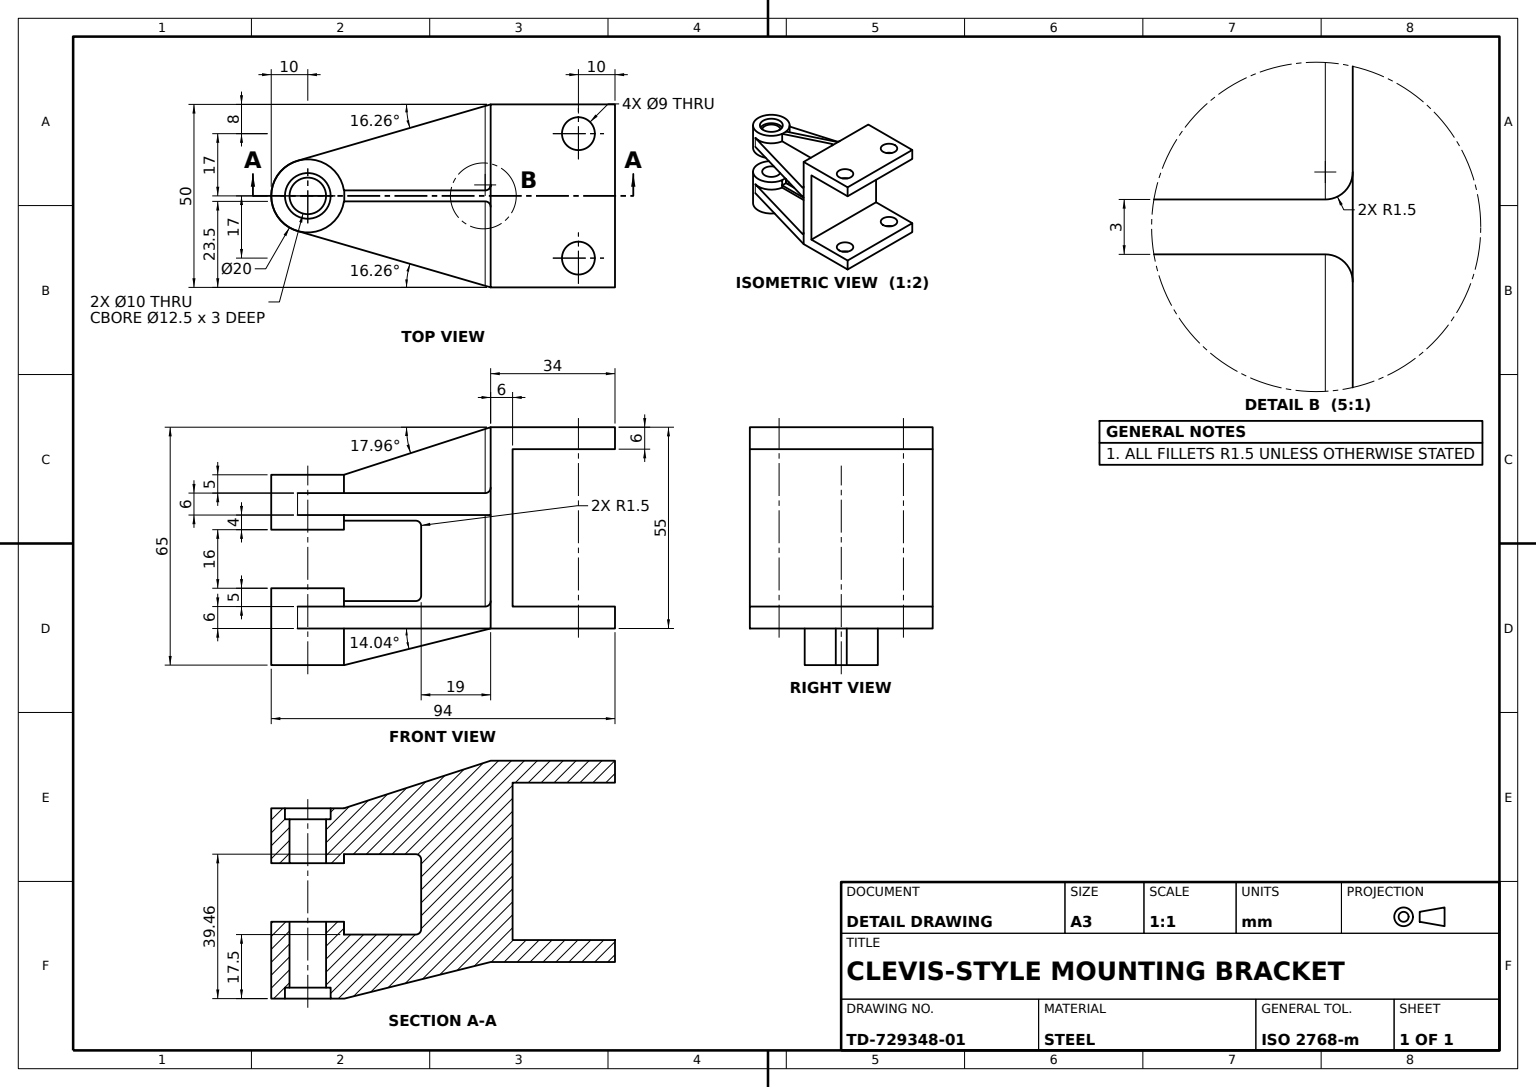
from build123d import *

# Parameters (mm, degrees)
U_CHANNEL_BASE_DEPTH             = 25
UPPER_LUG_BOSS_SKETCH_20_R       = 10
UPPER_LUG_BOSS_20_DEPTH          = 10
UPPER_START                      = 5
UPPER_LUG_PAD_SKETCH_R           = 10
UPPER_LUG_PAD_DEPTH              = 5
UPPER_COUNTERBORE_SKETCH_12_5_R  = 6.25
UPPER_COUNTERBORE_12_5_DEPTH     = 3
UPPER_LUG_HOLE_SKETCH_10_R       = 5
UPPER_LUG_HOLE_10_DEPTH          = 12
LOWER_START                      = -11
LOWER_LUG_PAD_SKETCH_R           = 10
LOWER_LUG_PAD_DEPTH              = 11
LOWER_LUG_BOSS_SKETCH_20_R       = 10
LOWER_LUG_BOSS_20_DEPTH          = 10
LOWER_START_2                    = -3
LOWER_COUNTERBORE_SKETCH_12_5_R  = 6.25
LOWER_COUNTERBORE_12_5_DEPTH     = 3
LOWER_START_3                    = -18
LOWER_LUG_HOLE_SKETCH_10_R       = 5
LOWER_LUG_HOLE_10_DEPTH          = 18
UPPER_GUSSET_DEPTH               = 6
UPPER_GUSSET_TRIM_DEPTH          = 6
LOWER_GUSSET_DEPTH               = 6
LOWER_GUSSET_TRIM_DEPTH          = 6
BACK_PLATE_DEPTH                 = 1.5
BACK_PLATE_LOWER_RELIEF_DEPTH    = 3
LOWER_LUG_RELIEF_SKETCH_W        = 3
LOWER_LUG_RELIEF_SKETCH_H        = 5
LOWER_LUG_RELIEF_DEPTH           = 3
BACK_PLATE_UPPER_RELIEF_SKETCH_W = 40.123603225
BACK_PLATE_UPPER_RELIEF_SKETCH_H = 13
BACK_PLATE_UPPER_RELIEF_DEPTH    = 3
BACK_PLATE_EDGE_TRIM_SKETCH_W    = 21.123603225
BACK_PLATE_EDGE_TRIM_SKETCH_H    = 21.964107992
BACK_PLATE_EDGE_TRIM_DEPTH       = 3
WEB_SKETCH_W                     = 40.123603225
WEB_SKETCH_H                     = 3
WEB_DEPTH                        = 18
WEB_CHAMFER_CUT_DEPTH            = 3
WEB_FACE_TRIM_SKETCH_W           = 3
WEB_FACE_TRIM_SKETCH_H           = 13
WEB_FACE_TRIM_0_1_DEPTH          = 0.1
FLANGE_MOUNTING_HOLES_SKETCH_R   = 4.5
FLANGE_MOUNTING_HOLES_4X_DEPTH   = 59.1
EDGE_FILLET_R1_5_R               = 1.5


with BuildPart() as part:
    # U-Channel Profile Sketch → U-Channel Base (new, symmetric)
    with BuildSketch(Plane.XY):
        Polygon((0, 37.5), (0, 19.5), (-50, 19.5), (-50, 13.5), (0, 13.5), (0, -11.5), (-50, -11.5), (-50, -17.5), (0, -17.5), (34, -17.5), (34, -11.5), (6, -11.5), (6, 31.5), (34, 31.5), (34, 37.5), align=None)
    extrude(amount=U_CHANNEL_BASE_DEPTH, both=True)

    # Upper Lug Boss Sketch Ø20 → Upper Lug Boss Ø20 (add)
    with BuildSketch(Plane(origin=(0, 19.5, 0), x_dir=(1, 0, 0), z_dir=(0, 1, 0))):
        with Locations(Location((-50, 0, 0), (0, 0, 180))):
            Circle(UPPER_LUG_BOSS_SKETCH_20_R)
    extrude(amount=-UPPER_LUG_BOSS_20_DEPTH)

    # Upper Lug Pad Sketch → Upper Lug Pad (add)
    with BuildSketch(Plane(origin=(0, 19.5, 0), x_dir=(1, 0, 0), z_dir=(0, 1, 0)).offset(UPPER_START)):
        with Locations(Location((-50, 0, 0), (0, 0, 180))):
            Circle(UPPER_LUG_PAD_SKETCH_R)
    extrude(amount=-UPPER_LUG_PAD_DEPTH)

    # Upper Counterbore Sketch Ø12.5 → Upper Counterbore Ø12.5 (cut)
    with BuildSketch(Plane(origin=(0, 24.5, 0), x_dir=(1, 0, 0), z_dir=(0, 1, 0))):
        with Locations(Location((-50, 0, 0), (0, 0, 180))):
            Circle(UPPER_COUNTERBORE_SKETCH_12_5_R)
    extrude(amount=-UPPER_COUNTERBORE_12_5_DEPTH, mode=Mode.SUBTRACT)

    # Upper Lug Hole Sketch Ø10 → Upper Lug Hole Ø10 (cut)
    with BuildSketch(Plane(origin=(0, 21.5, 0), x_dir=(1, 0, 0), z_dir=(0, 1, 0))):
        with Locations(Location((-50, 0, 0), (0, 0, 180))):
            Circle(UPPER_LUG_HOLE_SKETCH_10_R)
    extrude(amount=-UPPER_LUG_HOLE_10_DEPTH, mode=Mode.SUBTRACT)

    # Lower Lug Pad Sketch → Lower Lug Pad (add)
    with BuildSketch(Plane.XZ.offset(17.5).offset(LOWER_START)):
        with Locations(Location((-50, 0, 0), (0, 0, 180))):
            Circle(LOWER_LUG_PAD_SKETCH_R)
    extrude(amount=LOWER_LUG_PAD_DEPTH)

    # Lower Lug Boss Sketch Ø20 → Lower Lug Boss Ø20 (add)
    with BuildSketch(Plane.XZ.offset(17.5)):
        with Locations(Location((-50, 0, 0), (0, 0, 180))):
            Circle(LOWER_LUG_BOSS_SKETCH_20_R)
    extrude(amount=LOWER_LUG_BOSS_20_DEPTH)

    # Lower Counterbore Sketch Ø12.5 → Lower Counterbore Ø12.5 (cut)
    with BuildSketch(Plane.XZ.offset(27.5).offset(LOWER_START_2)):
        with Locations(Location((-50, 0, 0), (0, 0, 180))):
            Circle(LOWER_COUNTERBORE_SKETCH_12_5_R)
    extrude(amount=LOWER_COUNTERBORE_12_5_DEPTH, mode=Mode.SUBTRACT)

    # Lower Lug Hole Sketch Ø10 → Lower Lug Hole Ø10 (cut)
    with BuildSketch(Plane.XZ.offset(24.5).offset(LOWER_START_3)):
        with Locations(Location((-50, 0, 0), (0, 0, 180))):
            Circle(LOWER_LUG_HOLE_SKETCH_10_R)
    extrude(amount=LOWER_LUG_HOLE_10_DEPTH, mode=Mode.SUBTRACT)

    # Upper Gusset Sketch → Upper Gusset (add)
    with BuildSketch(Plane(origin=(0, 19.5, 0), x_dir=(1, 0, 0), z_dir=(0, 1, 0))):
        Polygon((0, 25), (-50, 10.416666667), (-50, 10), (-52.8, 9.6), (-52.8, 25), align=None)
        Polygon((-52.8, -9.6), (-52.8, -25), (0, -25), (-50, -10.416666667), (-50, -10), align=None)
    extrude(amount=-UPPER_GUSSET_DEPTH)

    # Upper Gusset Trim Sketch → Upper Gusset Trim (cut)
    with BuildSketch(Plane(origin=(0, 19.5, 0), x_dir=(1, 0, 0), z_dir=(0, 1, 0))):
        Polygon((0, 25), (-52.8, 9.6), (-52.8, 25), align=None)
        Polygon((0, -25), (-52.8, -9.6), (-52.8, -25), align=None)
    extrude(amount=-UPPER_GUSSET_TRIM_DEPTH, mode=Mode.SUBTRACT)

    # Lower Gusset Sketch → Lower Gusset (add)
    with BuildSketch(Plane.XZ.offset(17.5)):
        Polygon((0, 25), (-50, 10.416666667), (-50, 10), (-52.8, 9.6), (-52.8, 25), align=None)
        Polygon((0, -25), (-50, -10.416666667), (-50, -10), (-52.8, -9.6), (-52.8, -25), align=None)
    extrude(amount=-LOWER_GUSSET_DEPTH)

    # Lower Gusset Trim Sketch → Lower Gusset Trim (cut)
    with BuildSketch(Plane.XZ.offset(17.5)):
        Polygon((0, 25), (-52.8, 9.6), (-52.8, 25), align=None)
        Polygon((0, -25), (-52.8, -9.6), (-52.8, -25), align=None)
    extrude(amount=-LOWER_GUSSET_TRIM_DEPTH, mode=Mode.SUBTRACT)


with BuildPart() as body_2:
    # Back Plate Sketch → Back Plate (new, symmetric)
    with BuildSketch(Plane.XY):
        Polygon((0, 0), (0, 32.5), (-40.123603225, 32.5), (-40.123603225, -32.5), (0, -32.5), align=None)
    extrude(amount=BACK_PLATE_DEPTH, both=True)

    # Back Plate Lower Relief Sketch → Back Plate Lower Relief (cut)
    with BuildSketch(Plane.XY.offset(1.5)):
        Polygon((-40, -27.5), (0, -17.5), (0, -32.5), (-40.123603225, -32.5), align=None)
    extrude(amount=-BACK_PLATE_LOWER_RELIEF_DEPTH, mode=Mode.SUBTRACT)

    # Lower Lug Relief Sketch → Lower Lug Relief (cut)
    with BuildSketch(Plane.ZY.offset(40.123603225)):
        with Locations((0, -30)):
            Rectangle(LOWER_LUG_RELIEF_SKETCH_W, LOWER_LUG_RELIEF_SKETCH_H)
    extrude(amount=-LOWER_LUG_RELIEF_DEPTH, mode=Mode.SUBTRACT)


with BuildPart() as back_plate_upper_relief_tool:
    # Back Plate Upper Relief Sketch → Back Plate Upper Relief (new body)
    with BuildSketch(Plane.XY.offset(1.5)):
        with Locations((-20.061801613, 26)):
            Rectangle(BACK_PLATE_UPPER_RELIEF_SKETCH_W, BACK_PLATE_UPPER_RELIEF_SKETCH_H)
    extrude(amount=-BACK_PLATE_UPPER_RELIEF_DEPTH)


with BuildPart() as part_1:
    add(part.part)

    # Back Plate Upper Relief: cut by back_plate_upper_relief_tool
    add(back_plate_upper_relief_tool.part, mode=Mode.SUBTRACT)


with BuildPart() as body_2_1:
    add(body_2.part)

    # Back Plate Upper Relief: cut by back_plate_upper_relief_tool
    add(back_plate_upper_relief_tool.part, mode=Mode.SUBTRACT)


with BuildPart() as back_plate_edge_trim_tool:
    # Back Plate Edge Trim Sketch → Back Plate Edge Trim (new body)
    with BuildSketch(Plane.XY.offset(1.5)):
        with Locations((-29.561801613, 0.982053996)):
            Rectangle(BACK_PLATE_EDGE_TRIM_SKETCH_W, BACK_PLATE_EDGE_TRIM_SKETCH_H)
    extrude(amount=-BACK_PLATE_EDGE_TRIM_DEPTH)


with BuildPart() as part_2:
    add(part_1.part)

    # Back Plate Edge Trim: cut by back_plate_edge_trim_tool
    add(back_plate_edge_trim_tool.part, mode=Mode.SUBTRACT)



with BuildPart() as body_2_2:
    add(body_2_1.part)

    # Back Plate Edge Trim: cut by back_plate_edge_trim_tool
    add(back_plate_edge_trim_tool.part, mode=Mode.SUBTRACT)


with BuildPart() as part_3:
    add(part_2.part)

    add(body_2_2.part)  # Web merges body 2
    # Web Sketch → Web (add)
    with BuildSketch(Plane(origin=(0, 19.5, 0), x_dir=(1, 0, 0), z_dir=(0, 1, 0))):
        with Locations((-20.061801613, 0)):
            Rectangle(WEB_SKETCH_W, WEB_SKETCH_H)
    extrude(amount=WEB_DEPTH)

    # Web Chamfer Cut Sketch → Web Chamfer Cut (cut)
    with BuildSketch(Plane.XY.offset(1.5)):
        Polygon((0, 37.5), (-40.113140033, 24.5), (-40.123603225, 37.5), align=None)
    extrude(amount=-WEB_CHAMFER_CUT_DEPTH, mode=Mode.SUBTRACT)

    # Web Face Trim Sketch → Web Face Trim 0.1 (cut)
    with BuildSketch(Plane.ZY.offset(40.123603225)):
        with Locations((0, 31)):
            Rectangle(WEB_FACE_TRIM_SKETCH_W, WEB_FACE_TRIM_SKETCH_H)
    extrude(amount=-WEB_FACE_TRIM_0_1_DEPTH, mode=Mode.SUBTRACT)

    # Flange Mounting Holes Sketch → Flange Mounting Holes 4x (cut)
    with BuildSketch(Plane(origin=(0, 37.5, 0), x_dir=(1, 0, 0), z_dir=(0, 1, 0))):
        with Locations(Location((24, 17, 0), (0, 0, 270))):
            Circle(FLANGE_MOUNTING_HOLES_SKETCH_R)
        with Locations(Location((24, -17, 0), (0, 0, 270))):
            Circle(FLANGE_MOUNTING_HOLES_SKETCH_R)
    extrude(amount=-FLANGE_MOUNTING_HOLES_4X_DEPTH, mode=Mode.SUBTRACT)

    # Edge Fillet R1.5
    edge_fillet_r1_5_edges = [part_3.edges().sort_by_distance(p)[0] for p in [
        (0, -11.5, 13.25),
        (0, 19.5, 13.25),
        (0, 19.5, -13.25),
        (0, 28.5, 1.5),
        (0, 28.5, -1.5),
        (0, -11.5, -13.25),
        (0, 1, -1.5),
        (0, 1, 1.5),
        (-19, 11.964107992, 0),
        (-19, -10, 0),
    ]]
    fillet(edge_fillet_r1_5_edges, radius=EDGE_FILLET_R1_5_R)


solid = part_3.part
